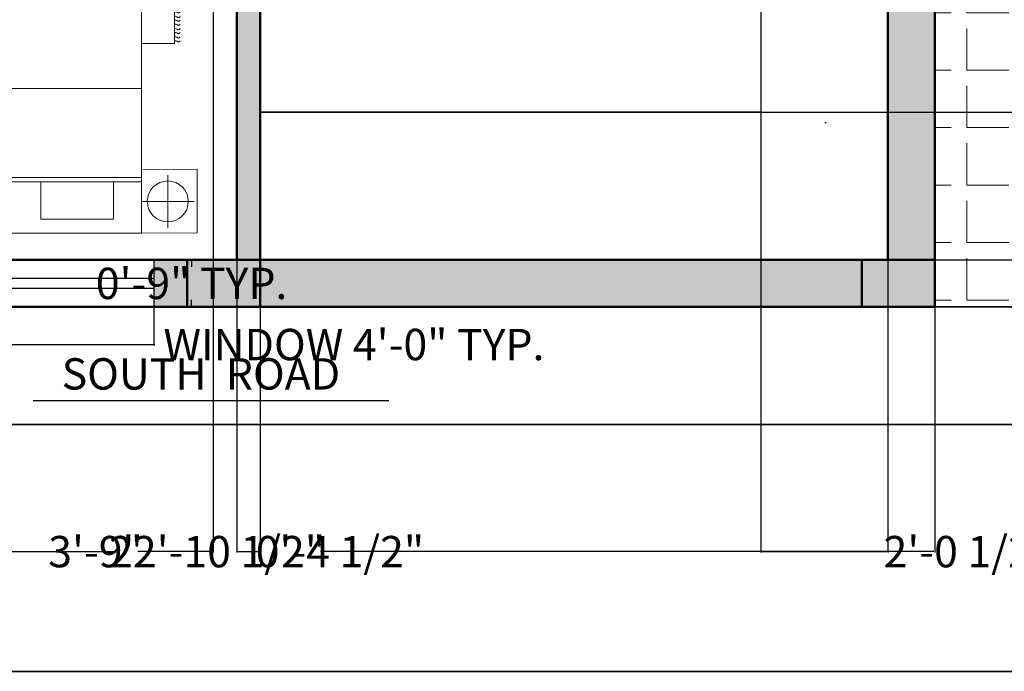
# Model space of a CAD drawing. Units: inches. Extents: x 1601 to 2080, y 5000 to 5589.
# Tile 3 of 11: x 1788 to 1976, y 5000 to 5125. Entities that reach past the tile are written whole.
import ezdxf

# ---------------------------------------------------------------- set-up
doc = ezdxf.new("R2010")
doc.units = ezdxf.units.IN
doc.header["$MEASUREMENT"] = 0
for name, color, linetype, lineweight in [('A-ANNO-DIMS', 2, 'Continuous', 18), ('A-ANNO-TEXT', 7, 'Continuous', 25), ('A-ANNO-TTLB', 7, 'Continuous', 35), ('A-COLS', 7, 'Continuous', 50), ('A-COLS-PATT', 18, 'Continuous', 13), ('A-FLOR-CASE', 8, 'Continuous', 25), ('A-FLOR-PATT', 8, 'Continuous', 13), ('A-FURN', 8, 'Continuous', 18), ('A-GLAZ', 4, 'Continuous', 25), ('A-WALL', 7, 'Continuous', 50), ('A-WALL-PATT', 241, 'Continuous', 13), ('C-PROP', 7, 'Continuous', 35)]:
    doc.layers.add(name, color=color, linetype=linetype, lineweight=lineweight)
doc.styles.get("Standard").update_dxf_attribs({"font": 'arial.ttf'})
doc.dimstyles.get("Standard").update_dxf_attribs({"dimtxt": 6, "dimasz": 0.18, "dimexe": 0.18, "dimexo": 0.0625, "dimgap": 0.09, "dimtad": 0, "dimtih": 1, "dimtoh": 1, "dimdec": 1, "dimzin": 0, "dimdsep": 46, "dimlunit": 3, "dimtxsty": 'Standard', "dimcen": 0.09, "dimadec": 0, "dimazin": 0, "dimtfac": 1, "dimtdec": 1, "dimtofl": 0, "dimtmove": 0, "dimatfit": 3, "dimfxl": 1, "dimtolj": 1, "dimtzin": 0, "dimarcsym": 0})

# ---------------------------------------------------------------- blocks, each defined once
blk = doc.blocks.new('BED-DOUBLE-ENSEMBLE')
for p, q in [((5.6, 61.61), (5.6, 51.56)), ((63.65, 61.72), (63.65, 51.66)), ((10.63, 56.59), (0.57, 56.59)), ((68.68, 56.69), (58.62, 56.69)), ((49.39, 52.82), (10.63, 52.82)), ((49.39, 52.82), (58, 46.47)), ((49.44, 52.82), (49.44, 46.47)), ((49.44, 52), (10.63, 52)), ((49.44, 46.47), (58, 46.47)), ((58.05, 34.96), (10.63, 34.96)), ((4.35, 0), (4.35, 26.37)), ((4.35, 26.37), (10.65, 26.37)), ((58.05, 26.37), (67.59, 26.37)), ((67.59, 26.37), (67.59, 0)), ((67.59, 0), (4.35, 0))]:
    blk.add_line(p, q)
for points in [[(0, 50.39), (10.63, 50.5), (10.63, 62.68), (0, 62.58)], [(58.05, 62.68), (58.05, 11.36), (10.63, 11.36), (10.63, 62.68)], [(58.05, 50.5), (68.68, 50.6), (68.68, 62.78), (58.05, 62.68)], [(29.88, 59.98), (29.88, 52.82), (15.98, 52.82), (15.98, 59.98)], [(49.44, 59.98), (49.44, 52.82), (35.55, 52.82), (35.55, 59.98)]]:
    blk.add_lwpolyline(points, close=True)
for centre in [(5.6, 56.59), (63.65, 56.69)]:
    blk.add_circle(centre, 3.92)
for points, knots in [([(3.23, 25.83), (3.32, 25.96), (3.52, 26.2), (3.86, 25.96), (4.14, 25.78), (4.29, 25.89), (4.35, 25.94)], [0, 0, 0, 0, 0.400747, 0.791423, 1.067667, 1.29709, 1.29709, 1.29709, 1.29709]), ([(3.23, 25.06), (3.32, 25.18), (3.52, 25.42), (3.86, 25.18), (4.14, 25), (4.29, 25.11), (4.35, 25.16)], [0, 0, 0, 0, 0.400747, 0.791423, 1.067667, 1.29709, 1.29709, 1.29709, 1.29709]), ([(3.23, 24.24), (3.32, 24.36), (3.52, 24.6), (3.86, 24.36), (4.14, 24.19), (4.29, 24.3), (4.35, 24.34)], [0, 0, 0, 0, 0.400747, 0.791423, 1.067667, 1.29709, 1.29709, 1.29709, 1.29709]), ([(68.71, 25.83), (68.61, 25.96), (68.42, 26.2), (68.08, 25.96), (67.8, 25.78), (67.65, 25.89), (67.58, 25.94)], [0, 0, 0, 0, 0.400747, 0.791423, 1.067667, 1.29709, 1.29709, 1.29709, 1.29709]), ([(68.71, 25.06), (68.61, 25.18), (68.42, 25.42), (68.08, 25.18), (67.8, 25), (67.65, 25.11), (67.58, 25.16)], [0, 0, 0, 0, 0.400747, 0.791423, 1.067667, 1.29709, 1.29709, 1.29709, 1.29709]), ([(68.71, 24.24), (68.61, 24.36), (68.42, 24.6), (68.08, 24.36), (67.8, 24.19), (67.65, 24.3), (67.58, 24.34)], [0, 0, 0, 0, 0.400747, 0.791423, 1.067667, 1.29709, 1.29709, 1.29709, 1.29709]), ([(3.23, 23.51), (3.32, 23.63), (3.52, 23.87), (3.86, 23.63), (4.14, 23.46), (4.29, 23.57), (4.35, 23.62)], [0, 0, 0, 0, 0.400747, 0.791423, 1.067667, 1.29709, 1.29709, 1.29709, 1.29709]), ([(3.23, 22.63), (3.32, 22.75), (3.52, 22.99), (3.86, 22.75), (4.14, 22.58), (4.29, 22.68), (4.35, 22.73)], [0, 0, 0, 0, 0.400747, 0.791423, 1.067667, 1.29709, 1.29709, 1.29709, 1.29709]), ([(68.71, 23.51), (68.61, 23.63), (68.42, 23.87), (68.08, 23.63), (67.8, 23.46), (67.65, 23.57), (67.58, 23.62)], [0, 0, 0, 0, 0.400747, 0.791423, 1.067667, 1.29709, 1.29709, 1.29709, 1.29709]), ([(68.71, 22.63), (68.61, 22.75), (68.42, 22.99), (68.08, 22.75), (67.8, 22.58), (67.65, 22.68), (67.58, 22.73)], [0, 0, 0, 0, 0.400747, 0.791423, 1.067667, 1.29709, 1.29709, 1.29709, 1.29709]), ([(3.23, 21.88), (3.32, 22), (3.52, 22.24), (3.86, 22), (4.14, 21.83), (4.29, 21.93), (4.35, 21.98)], [0, 0, 0, 0, 0.400747, 0.791423, 1.067667, 1.29709, 1.29709, 1.29709, 1.29709]), ([(3.23, 21.15), (3.32, 21.27), (3.52, 21.51), (3.86, 21.27), (4.14, 21.1), (4.29, 21.2), (4.35, 21.25)], [0, 0, 0, 0, 0.400747, 0.791423, 1.067667, 1.29709, 1.29709, 1.29709, 1.29709]), ([(68.71, 21.88), (68.61, 22), (68.42, 22.24), (68.08, 22), (67.8, 21.83), (67.65, 21.93), (67.58, 21.98)], [0, 0, 0, 0, 0.400747, 0.791423, 1.067667, 1.29709, 1.29709, 1.29709, 1.29709]), ([(68.71, 21.15), (68.61, 21.27), (68.42, 21.51), (68.08, 21.27), (67.8, 21.1), (67.65, 21.2), (67.58, 21.25)], [0, 0, 0, 0, 0.400747, 0.791423, 1.067667, 1.29709, 1.29709, 1.29709, 1.29709]), ([(3.23, 20.27), (3.32, 20.39), (3.52, 20.63), (3.86, 20.39), (4.14, 20.22), (4.29, 20.32), (4.35, 20.37)], [0, 0, 0, 0, 0.400747, 0.791423, 1.067667, 1.29709, 1.29709, 1.29709, 1.29709]), ([(3.23, 19.23), (3.32, 19.35), (3.52, 19.59), (3.86, 19.35), (4.14, 19.18), (4.29, 19.29), (4.35, 19.33)], [0, 0, 0, 0, 0.400747, 0.791423, 1.067667, 1.29709, 1.29709, 1.29709, 1.29709]), ([(68.71, 20.27), (68.61, 20.39), (68.42, 20.63), (68.08, 20.39), (67.8, 20.22), (67.65, 20.32), (67.58, 20.37)], [0, 0, 0, 0, 0.400747, 0.791423, 1.067667, 1.29709, 1.29709, 1.29709, 1.29709]), ([(68.71, 19.23), (68.61, 19.35), (68.42, 19.59), (68.08, 19.35), (67.8, 19.18), (67.65, 19.29), (67.58, 19.33)], [0, 0, 0, 0, 0.400747, 0.791423, 1.067667, 1.29709, 1.29709, 1.29709, 1.29709]), ([(3.23, 18.35), (3.32, 18.47), (3.52, 18.71), (3.86, 18.47), (4.14, 18.3), (4.29, 18.4), (4.35, 18.45)], [0, 0, 0, 0, 0.400747, 0.791423, 1.067667, 1.29709, 1.29709, 1.29709, 1.29709]), ([(3.23, 17.53), (3.32, 17.65), (3.52, 17.89), (3.86, 17.65), (4.14, 17.48), (4.29, 17.59), (4.35, 17.64)], [0, 0, 0, 0, 0.400747, 0.791423, 1.067667, 1.29709, 1.29709, 1.29709, 1.29709]), ([(3.23, 16.76), (3.32, 16.88), (3.52, 17.12), (3.86, 16.88), (4.14, 16.7), (4.29, 16.81), (4.35, 16.86)], [0, 0, 0, 0, 0.400747, 0.791423, 1.067667, 1.29709, 1.29709, 1.29709, 1.29709]), ([(68.71, 18.35), (68.61, 18.47), (68.42, 18.71), (68.08, 18.47), (67.8, 18.3), (67.65, 18.4), (67.58, 18.45)], [0, 0, 0, 0, 0.400747, 0.791423, 1.067667, 1.29709, 1.29709, 1.29709, 1.29709]), ([(68.71, 17.53), (68.61, 17.65), (68.42, 17.89), (68.08, 17.65), (67.8, 17.48), (67.65, 17.59), (67.58, 17.64)], [0, 0, 0, 0, 0.400747, 0.791423, 1.067667, 1.29709, 1.29709, 1.29709, 1.29709]), ([(68.71, 16.76), (68.61, 16.88), (68.42, 17.12), (68.08, 16.88), (67.8, 16.7), (67.65, 16.81), (67.58, 16.86)], [0, 0, 0, 0, 0.400747, 0.791423, 1.067667, 1.29709, 1.29709, 1.29709, 1.29709]), ([(3.23, 15.94), (3.32, 16.06), (3.52, 16.3), (3.86, 16.06), (4.14, 15.89), (4.29, 15.99), (4.35, 16.04)], [0, 0, 0, 0, 0.400747, 0.791423, 1.067667, 1.29709, 1.29709, 1.29709, 1.29709]), ([(3.23, 15.21), (3.32, 15.33), (3.52, 15.57), (3.86, 15.33), (4.14, 15.16), (4.29, 15.27), (4.35, 15.31)], [0, 0, 0, 0, 0.400747, 0.791423, 1.067667, 1.29709, 1.29709, 1.29709, 1.29709]), ([(68.71, 15.94), (68.61, 16.06), (68.42, 16.3), (68.08, 16.06), (67.8, 15.89), (67.65, 15.99), (67.58, 16.04)], [0, 0, 0, 0, 0.400747, 0.791423, 1.067667, 1.29709, 1.29709, 1.29709, 1.29709]), ([(68.71, 15.21), (68.61, 15.33), (68.42, 15.57), (68.08, 15.33), (67.8, 15.16), (67.65, 15.27), (67.58, 15.31)], [0, 0, 0, 0, 0.400747, 0.791423, 1.067667, 1.29709, 1.29709, 1.29709, 1.29709]), ([(3.23, 14.33), (3.32, 14.45), (3.52, 14.69), (3.86, 14.45), (4.14, 14.28), (4.29, 14.38), (4.35, 14.43)], [0, 0, 0, 0, 0.400747, 0.791423, 1.067667, 1.29709, 1.29709, 1.29709, 1.29709]), ([(3.23, 13.58), (3.32, 13.7), (3.52, 13.94), (3.86, 13.7), (4.14, 13.53), (4.29, 13.63), (4.35, 13.68)], [0, 0, 0, 0, 0.400747, 0.791423, 1.067667, 1.29709, 1.29709, 1.29709, 1.29709]), ([(68.71, 14.33), (68.61, 14.45), (68.42, 14.69), (68.08, 14.45), (67.8, 14.28), (67.65, 14.38), (67.58, 14.43)], [0, 0, 0, 0, 0.400747, 0.791423, 1.067667, 1.29709, 1.29709, 1.29709, 1.29709]), ([(68.71, 13.58), (68.61, 13.7), (68.42, 13.94), (68.08, 13.7), (67.8, 13.53), (67.65, 13.63), (67.58, 13.68)], [0, 0, 0, 0, 0.400747, 0.791423, 1.067667, 1.29709, 1.29709, 1.29709, 1.29709]), ([(3.23, 12.85), (3.32, 12.97), (3.52, 13.21), (3.86, 12.97), (4.14, 12.8), (4.29, 12.9), (4.35, 12.95)], [0, 0, 0, 0, 0.400747, 0.791423, 1.067667, 1.29709, 1.29709, 1.29709, 1.29709]), ([(3.23, 11.97), (3.32, 12.09), (3.52, 12.33), (3.86, 12.09), (4.14, 11.92), (4.29, 12.02), (4.35, 12.07)], [0, 0, 0, 0, 0.400747, 0.791423, 1.067667, 1.29709, 1.29709, 1.29709, 1.29709]), ([(68.71, 12.85), (68.61, 12.97), (68.42, 13.21), (68.08, 12.97), (67.8, 12.8), (67.65, 12.9), (67.58, 12.95)], [0, 0, 0, 0, 0.400747, 0.791423, 1.067667, 1.29709, 1.29709, 1.29709, 1.29709]), ([(68.71, 11.97), (68.61, 12.09), (68.42, 12.33), (68.08, 12.09), (67.8, 11.92), (67.65, 12.02), (67.58, 12.07)], [0, 0, 0, 0, 0.400747, 0.791423, 1.067667, 1.29709, 1.29709, 1.29709, 1.29709]), ([(3.23, 10.93), (3.32, 11.05), (3.52, 11.29), (3.86, 11.05), (4.14, 10.88), (4.29, 10.99), (4.35, 11.03)], [0, 0, 0, 0, 0.400747, 0.791423, 1.067667, 1.29709, 1.29709, 1.29709, 1.29709]), ([(3.23, 10.05), (3.32, 10.17), (3.52, 10.41), (3.86, 10.17), (4.14, 10), (4.29, 10.1), (4.35, 10.15)], [0, 0, 0, 0, 0.400747, 0.791423, 1.067667, 1.29709, 1.29709, 1.29709, 1.29709]), ([(3.23, 9.23), (3.32, 9.35), (3.52, 9.59), (3.86, 9.35), (4.14, 9.18), (4.29, 9.29), (4.35, 9.34)], [0, 0, 0, 0, 0.400747, 0.791423, 1.067667, 1.29709, 1.29709, 1.29709, 1.29709]), ([(68.71, 10.93), (68.61, 11.05), (68.42, 11.29), (68.08, 11.05), (67.8, 10.88), (67.65, 10.99), (67.58, 11.03)], [0, 0, 0, 0, 0.400747, 0.791423, 1.067667, 1.29709, 1.29709, 1.29709, 1.29709]), ([(68.71, 10.05), (68.61, 10.17), (68.42, 10.41), (68.08, 10.17), (67.8, 10), (67.65, 10.1), (67.58, 10.15)], [0, 0, 0, 0, 0.400747, 0.791423, 1.067667, 1.29709, 1.29709, 1.29709, 1.29709]), ([(68.71, 9.23), (68.61, 9.35), (68.42, 9.59), (68.08, 9.35), (67.8, 9.18), (67.65, 9.29), (67.58, 9.34)], [0, 0, 0, 0, 0.400747, 0.791423, 1.067667, 1.29709, 1.29709, 1.29709, 1.29709]), ([(3.23, 8.54), (3.32, 8.66), (3.52, 8.9), (3.86, 8.66), (4.14, 8.49), (4.29, 8.6), (4.35, 8.65)], [0, 0, 0, 0, 0.400747, 0.791423, 1.067667, 1.29709, 1.29709, 1.29709, 1.29709]), ([(3.23, 7.73), (3.32, 7.85), (3.52, 8.09), (3.86, 7.85), (4.14, 7.67), (4.29, 7.78), (4.35, 7.83)], [0, 0, 0, 0, 0.400747, 0.791423, 1.067667, 1.29709, 1.29709, 1.29709, 1.29709]), ([(68.71, 8.54), (68.61, 8.66), (68.42, 8.9), (68.08, 8.66), (67.8, 8.49), (67.65, 8.6), (67.58, 8.65)], [0, 0, 0, 0, 0.400747, 0.791423, 1.067667, 1.29709, 1.29709, 1.29709, 1.29709]), ([(68.71, 7.73), (68.61, 7.85), (68.42, 8.09), (68.08, 7.85), (67.8, 7.67), (67.65, 7.78), (67.58, 7.83)], [0, 0, 0, 0, 0.400747, 0.791423, 1.067667, 1.29709, 1.29709, 1.29709, 1.29709]), ([(3.23, 7), (3.32, 7.12), (3.52, 7.36), (3.86, 7.12), (4.14, 6.95), (4.29, 7.05), (4.35, 7.1)], [0, 0, 0, 0, 0.400747, 0.791423, 1.067667, 1.29709, 1.29709, 1.29709, 1.29709]), ([(3.23, 6.12), (3.32, 6.24), (3.52, 6.48), (3.86, 6.24), (4.14, 6.06), (4.29, 6.17), (4.35, 6.22)], [0, 0, 0, 0, 0.400747, 0.791423, 1.067667, 1.29709, 1.29709, 1.29709, 1.29709]), ([(68.71, 7), (68.61, 7.12), (68.42, 7.36), (68.08, 7.12), (67.8, 6.95), (67.65, 7.05), (67.58, 7.1)], [0, 0, 0, 0, 0.400747, 0.791423, 1.067667, 1.29709, 1.29709, 1.29709, 1.29709]), ([(68.71, 6.12), (68.61, 6.24), (68.42, 6.48), (68.08, 6.24), (67.8, 6.06), (67.65, 6.17), (67.58, 6.22)], [0, 0, 0, 0, 0.400747, 0.791423, 1.067667, 1.29709, 1.29709, 1.29709, 1.29709]), ([(3.23, 5.36), (3.32, 5.49), (3.52, 5.72), (3.86, 5.49), (4.14, 5.31), (4.29, 5.42), (4.35, 5.47)], [0, 0, 0, 0, 0.400747, 0.791423, 1.067667, 1.29709, 1.29709, 1.29709, 1.29709]), ([(3.23, 4.64), (3.32, 4.76), (3.52, 5), (3.86, 4.76), (4.14, 4.58), (4.29, 4.69), (4.35, 4.74)], [0, 0, 0, 0, 0.400747, 0.791423, 1.067667, 1.29709, 1.29709, 1.29709, 1.29709]), ([(3.23, 3.75), (3.32, 3.88), (3.52, 4.11), (3.86, 3.88), (4.14, 3.7), (4.29, 3.81), (4.35, 3.86)], [0, 0, 0, 0, 0.400747, 0.791423, 1.067667, 1.29709, 1.29709, 1.29709, 1.29709]), ([(68.71, 5.36), (68.61, 5.49), (68.42, 5.72), (68.08, 5.49), (67.8, 5.31), (67.65, 5.42), (67.58, 5.47)], [0, 0, 0, 0, 0.400747, 0.791423, 1.067667, 1.29709, 1.29709, 1.29709, 1.29709]), ([(68.71, 4.64), (68.61, 4.76), (68.42, 5), (68.08, 4.76), (67.8, 4.59), (67.66, 4.69), (67.59, 4.73)], [0, 0, 0, 0, 0.400747, 0.791423, 1.067667, 1.283686, 1.283686, 1.283686, 1.283686]), ([(68.71, 3.75), (68.61, 3.88), (68.42, 4.11), (68.08, 3.88), (67.8, 3.7), (67.66, 3.8), (67.59, 3.85)], [0, 0, 0, 0, 0.400747, 0.791423, 1.067667, 1.283686, 1.283686, 1.283686, 1.283686]), ([(3.23, 3.32), (3.32, 3.45), (3.51, 3.7), (3.86, 3.44), (4.14, 3.27), (4.29, 3.38), (4.35, 3.43)], [0, 0, 0, 0, 0.407265, 0.802015, 1.07826, 1.307683, 1.307683, 1.307683, 1.307683]), ([(3.23, 2.76), (3.32, 2.88), (3.52, 3.12), (3.86, 2.88), (4.14, 2.71), (4.29, 2.81), (4.35, 2.86)], [0, 0, 0, 0, 0.400747, 0.791423, 1.067667, 1.29709, 1.29709, 1.29709, 1.29709]), ([(3.23, 2.18), (3.32, 2.31), (3.52, 2.54), (3.86, 2.31), (4.14, 2.13), (4.29, 2.24), (4.35, 2.29)], [0, 0, 0, 0, 0.400747, 0.791423, 1.067667, 1.29709, 1.29709, 1.29709, 1.29709]), ([(3.23, 1.88), (3.32, 2), (3.52, 2.24), (3.86, 2), (4.14, 1.82), (4.29, 1.93), (4.35, 1.98)], [0, 0, 0, 0, 0.400747, 0.791423, 1.067667, 1.29709, 1.29709, 1.29709, 1.29709]), ([(68.71, 3.32), (68.61, 3.45), (68.42, 3.69), (68.08, 3.45), (67.8, 3.27), (67.66, 3.38), (67.59, 3.42)], [0, 0, 0, 0, 0.402903, 0.794912, 1.071156, 1.287177, 1.287177, 1.287177, 1.287177]), ([(68.71, 2.73), (68.61, 2.85), (68.42, 3.09), (68.08, 2.85), (67.8, 2.68), (67.66, 2.78), (67.59, 2.82)], [0, 0, 0, 0, 0.400747, 0.791423, 1.067667, 1.283686, 1.283686, 1.283686, 1.283686]), ([(68.71, 2.16), (68.61, 2.28), (68.42, 2.52), (68.08, 2.28), (67.8, 2.11), (67.66, 2.21), (67.59, 2.25)], [0, 0, 0, 0, 0.400747, 0.791423, 1.067667, 1.283686, 1.283686, 1.283686, 1.283686]), ([(68.71, 1.85), (68.61, 1.97), (68.42, 2.21), (68.08, 1.97), (67.8, 1.8), (67.66, 1.9), (67.59, 1.94)], [0, 0, 0, 0, 0.400747, 0.791423, 1.067667, 1.283686, 1.283686, 1.283686, 1.283686]), ([(3.23, 1.46), (3.32, 1.58), (3.52, 1.82), (3.86, 1.58), (4.14, 1.4), (4.29, 1.51), (4.35, 1.56)], [0, 0, 0, 0, 0.400747, 0.791423, 1.067667, 1.29709, 1.29709, 1.29709, 1.29709]), ([(3.23, 1.06), (3.32, 1.18), (3.52, 1.42), (3.86, 1.18), (4.14, 1.01), (4.29, 1.11), (4.35, 1.16)], [0, 0, 0, 0, 0.400747, 0.791423, 1.067667, 1.29709, 1.29709, 1.29709, 1.29709]), ([(3.23, 0.57), (3.32, 0.7), (3.52, 0.93), (3.86, 0.7), (4.14, 0.52), (4.29, 0.63), (4.35, 0.68)], [0, 0, 0, 0, 0.400747, 0.791423, 1.067667, 1.29709, 1.29709, 1.29709, 1.29709]), ([(3.23, 0.07), (3.32, 0.19), (3.52, 0.43), (3.86, 0.19), (4.14, 0.02), (4.29, 0.13), (4.35, 0.18)], [0, 0, 0, 0, 0.400747, 0.791423, 1.067667, 1.29709, 1.29709, 1.29709, 1.29709]), ([(68.71, 1.43), (68.61, 1.55), (68.42, 1.79), (68.08, 1.55), (67.8, 1.38), (67.65, 1.48), (67.58, 1.53)], [0, 0, 0, 0, 0.400747, 0.791423, 1.067667, 1.29709, 1.29709, 1.29709, 1.29709]), ([(68.71, 1.03), (68.61, 1.15), (68.42, 1.39), (68.08, 1.15), (67.8, 0.98), (67.65, 1.09), (67.58, 1.13)], [0, 0, 0, 0, 0.400747, 0.791423, 1.067667, 1.29709, 1.29709, 1.29709, 1.29709]), ([(68.71, 0.55), (68.61, 0.67), (68.42, 0.91), (68.08, 0.67), (67.8, 0.49), (67.65, 0.6), (67.58, 0.65)], [0, 0, 0, 0, 0.400747, 0.791423, 1.067667, 1.29709, 1.29709, 1.29709, 1.29709]), ([(68.71, 0.07), (68.61, 0.19), (68.42, 0.43), (68.08, 0.19), (67.8, 0.02), (67.65, 0.13), (67.58, 0.18)], [0, 0, 0, 0, 0.400747, 0.791423, 1.067667, 1.29709, 1.29709, 1.29709, 1.29709])]:
    blk.add_open_spline(points, degree=3, knots=knots)
blk = doc.blocks.new('WINDOW-48IN')
for p, q in [((0, 0), (0, 9)), ((0, 9), (48, 9)), ((48, 9), (48, 0)), ((0, 5.5), (48, 5.5)), ((48, 3.5), (0, 3.5)), ((48, 0), (0, 0))]:
    blk.add_line(p, q)
blk = doc.blocks.new('*D15')
at = {"layer": 'A-ANNO-DIMS', "color": 0, "lineweight": -2, "transparency": 16777216}
for p, q in [((1765.58, 5069.63), (1765.58, 5062.32)), ((1813.58, 5069.63), (1813.58, 5062.32)), ((1765.76, 5062.5), (1813.4, 5062.5)), ((1813.58, 5062.5), (1813.76, 5062.5))]:
    blk.add_line(p, q, dxfattribs=at)
at = {"layer": 'A-ANNO-DIMS', "color": 0, "transparency": 16777216}
for points in [[(1765.76, 5062.53), (1765.76, 5062.47), (1765.58, 5062.5)], [(1813.4, 5062.53), (1813.4, 5062.47), (1813.58, 5062.5)]]:
    blk.add_solid(points, dxfattribs=at)
at = {"layer": 'Defpoints', "color": 0, "transparency": 16777216}
for p in [(1765.58, 5069.7), (1813.58, 5069.7), (1813.58, 5062.5)]:
    blk.add_point(p, dxfattribs=at)
at = {"layer": 'A-ANNO-DIMS', "color": 0, "transparency": 16777216, "insert": (1851.82, 5062.5), "char_height": 6, "attachment_point": 5}
blk.add_mtext('\\A1;WINDOW 4\'-0" TYP.', dxfattribs=at)
blk = doc.blocks.new('*D16')
at = {"layer": 'A-ANNO-DIMS', "color": 0, "lineweight": -2, "transparency": 16777216}
for p, q in [((1813.65, 5078.7), (1820.96, 5078.7)), ((1820.78, 5078.52), (1820.78, 5077.35)), ((1820.78, 5069.88), (1820.78, 5071.04)), ((1813.65, 5069.7), (1820.96, 5069.7))]:
    blk.add_line(p, q, dxfattribs=at)
at = {"layer": 'A-ANNO-DIMS', "color": 0, "transparency": 16777216}
for points in [[(1820.75, 5078.52), (1820.81, 5078.52), (1820.78, 5078.7)], [(1820.75, 5069.88), (1820.81, 5069.88), (1820.78, 5069.7)]]:
    blk.add_solid(points, dxfattribs=at)
at = {"layer": 'Defpoints', "color": 0, "transparency": 16777216}
for p in [(1813.58, 5078.7), (1820.78, 5078.7), (1813.58, 5069.7)]:
    blk.add_point(p, dxfattribs=at)
at = {"layer": 'A-ANNO-DIMS', "color": 0, "transparency": 16777216, "insert": (1820.78, 5074.2), "char_height": 6, "attachment_point": 5}
blk.add_mtext('\\A1;0\'-9" TYP.', dxfattribs=at)
blk = doc.blocks.new('*D37')
at = {"layer": 'A-ANNO-DIMS', "color": 0, "lineweight": -2, "transparency": 16777216}
for p, q in [((1688.41, 5069.63), (1688.41, 5022.68)), ((1962.91, 5069.63), (1962.91, 5022.68)), ((1688.59, 5022.86), (1805.89, 5022.86)), ((1962.73, 5022.86), (1845.43, 5022.86))]:
    blk.add_line(p, q, dxfattribs=at)
at = {"layer": 'A-ANNO-DIMS', "color": 0, "transparency": 16777216}
for points in [[(1688.59, 5022.89), (1688.59, 5022.83), (1688.41, 5022.86)], [(1962.73, 5022.89), (1962.73, 5022.83), (1962.91, 5022.86)]]:
    blk.add_solid(points, dxfattribs=at)
at = {"layer": 'Defpoints', "color": 0, "transparency": 16777216}
for p in [(1688.41, 5069.7), (1962.91, 5069.7), (1962.91, 5022.86)]:
    blk.add_point(p, dxfattribs=at)
at = {"layer": 'A-ANNO-DIMS', "color": 0, "transparency": 16777216, "insert": (1825.66, 5022.86), "char_height": 6, "attachment_point": 5}
blk.add_mtext('\\A1;22\'-10 1/2"', dxfattribs=at)
blk = doc.blocks.new('*D44')
at = {"layer": 'A-ANNO-DIMS', "color": 0, "lineweight": -2, "transparency": 16777216}
for p, q in [((1929.65, 5106.89), (1929.65, 5022.68)), ((1953.91, 5078.63), (1953.91, 5022.68)), ((1929.83, 5022.86), (1953.73, 5022.86)), ((1953.91, 5022.86), (1954.09, 5022.86))]:
    blk.add_line(p, q, dxfattribs=at)
at = {"layer": 'A-ANNO-DIMS', "color": 0, "transparency": 16777216}
for points in [[(1929.83, 5022.89), (1929.83, 5022.83), (1929.65, 5022.86)], [(1953.73, 5022.89), (1953.73, 5022.83), (1953.91, 5022.86)]]:
    blk.add_solid(points, dxfattribs=at)
at = {"layer": 'Defpoints', "color": 0, "transparency": 16777216}
for p in [(1929.65, 5106.95), (1953.91, 5078.7), (1953.91, 5022.86)]:
    blk.add_point(p, dxfattribs=at)
at = {"layer": 'A-ANNO-DIMS', "color": 0, "transparency": 16777216, "insert": (1969.19, 5022.86), "char_height": 6, "attachment_point": 5}
blk.add_mtext('\\A1;2\'-0 1/2"', dxfattribs=at)
blk = doc.blocks.new('*D45')
at = {"layer": 'A-ANNO-DIMS', "color": 0, "lineweight": -2, "transparency": 16777216}
for p, q in [((1833.97, 5106.95), (2047.44, 5106.95)), ((2047.26, 5106.77), (2047.26, 5096.02)), ((2047.26, 5078.88), (2047.26, 5089.63)), ((1829.47, 5078.7), (2047.44, 5078.7))]:
    blk.add_line(p, q, dxfattribs=at)
at = {"layer": 'A-ANNO-DIMS', "color": 0, "transparency": 16777216}
for points in [[(2047.23, 5106.77), (2047.29, 5106.77), (2047.26, 5106.95)], [(2047.23, 5078.88), (2047.29, 5078.88), (2047.26, 5078.7)]]:
    blk.add_solid(points, dxfattribs=at)
at = {"layer": 'Defpoints', "color": 0, "transparency": 16777216}
for p in [(1833.91, 5106.95), (2047.26, 5106.95), (1829.41, 5078.7)]:
    blk.add_point(p, dxfattribs=at)
at = {"layer": 'A-ANNO-DIMS', "color": 0, "transparency": 16777216, "insert": (2047.26, 5092.83), "char_height": 6, "attachment_point": 5}
blk.add_mtext('\\A1;2\'-4 1/2"', dxfattribs=at)
blk = doc.blocks.new('*D50')
at = {"layer": 'A-ANNO-DIMS', "color": 0, "lineweight": -2, "transparency": 16777216}
for p, q in [((1962.97, 5136.6), (2047.44, 5136.6)), ((2047.26, 5136.42), (2047.26, 5106.29)), ((2047.26, 5069.88), (2047.26, 5100.01)), ((1962.97, 5069.7), (2047.44, 5069.7))]:
    blk.add_line(p, q, dxfattribs=at)
at = {"layer": 'A-ANNO-DIMS', "color": 0, "transparency": 16777216}
for points in [[(2047.23, 5136.42), (2047.29, 5136.42), (2047.26, 5136.6)], [(2047.23, 5069.88), (2047.29, 5069.88), (2047.26, 5069.7)]]:
    blk.add_solid(points, dxfattribs=at)
at = {"layer": 'Defpoints', "color": 0, "transparency": 16777216}
for p in [(1962.91, 5136.6), (2047.26, 5136.6), (1962.91, 5069.7)]:
    blk.add_point(p, dxfattribs=at)
at = {"layer": 'A-ANNO-DIMS', "color": 0, "transparency": 16777216, "insert": (2047.26, 5103.15), "char_height": 6, "attachment_point": 5}
blk.add_mtext('\\A1;5\'-7"', dxfattribs=at)
blk = doc.blocks.new('*D57')
at = {"layer": 'A-ANNO-DIMS', "color": 0, "lineweight": -2, "transparency": 16777216}
for p, q in [((1829.41, 5244.58), (1829.41, 5022.68)), ((1833.91, 5244.58), (1833.91, 5022.68)), ((1829.59, 5022.86), (1833.73, 5022.86)), ((1833.91, 5022.86), (1834.09, 5022.86))]:
    blk.add_line(p, q, dxfattribs=at)
at = {"layer": 'A-ANNO-DIMS', "color": 0, "transparency": 16777216}
for points in [[(1829.59, 5022.89), (1829.59, 5022.83), (1829.41, 5022.86)], [(1833.73, 5022.89), (1833.73, 5022.83), (1833.91, 5022.86)]]:
    blk.add_solid(points, dxfattribs=at)
at = {"layer": 'Defpoints', "color": 0, "transparency": 16777216}
for p in [(1829.41, 5244.64), (1833.91, 5244.64), (1833.91, 5022.86)]:
    blk.add_point(p, dxfattribs=at)
at = {"layer": 'A-ANNO-DIMS', "color": 0, "transparency": 16777216, "insert": (1849.14, 5022.86), "char_height": 6, "attachment_point": 5}
blk.add_mtext('\\A1;0\'-4 1/2"', dxfattribs=at)
blk = doc.blocks.new('*D58')
at = {"layer": 'A-ANNO-DIMS', "color": 0, "lineweight": -2, "transparency": 16777216}
for p, q in [((1779.91, 5209.13), (1779.91, 5022.68)), ((1824.91, 5209.13), (1824.91, 5022.68)), ((1780.09, 5022.86), (1794.35, 5022.86)), ((1824.73, 5022.86), (1810.47, 5022.86))]:
    blk.add_line(p, q, dxfattribs=at)
at = {"layer": 'A-ANNO-DIMS', "color": 0, "transparency": 16777216}
for points in [[(1780.09, 5022.89), (1780.09, 5022.83), (1779.91, 5022.86)], [(1824.73, 5022.89), (1824.73, 5022.83), (1824.91, 5022.86)]]:
    blk.add_solid(points, dxfattribs=at)
at = {"layer": 'Defpoints', "color": 0, "transparency": 16777216}
for p in [(1779.91, 5209.2), (1824.91, 5209.2), (1824.91, 5022.86)]:
    blk.add_point(p, dxfattribs=at)
at = {"layer": 'A-ANNO-DIMS', "color": 0, "transparency": 16777216, "insert": (1802.41, 5022.86), "char_height": 6, "attachment_point": 5}
blk.add_mtext('\\A1;3\'-9"', dxfattribs=at)
blk = doc.blocks.new('*D64')
at = {"layer": 'A-ANNO-DIMS', "color": 0, "lineweight": -2, "transparency": 16777216}
for p, q in [((1941.65, 5182.17), (1941.83, 5182.17)), ((1941.83, 5182.17), (1941.89, 5153.4)), ((1941.91, 5104.96), (1942.09, 5104.96)), ((1942, 5104.87), (1942, 5105.05))]:
    blk.add_line(p, q, dxfattribs=at)
at = {"layer": 'A-ANNO-DIMS', "color": 0, "transparency": 16777216}
blk.add_solid([(1941.92, 5153.4), (1941.86, 5153.4), (1941.89, 5153.22)], dxfattribs=at)
at = {"layer": 'Defpoints', "color": 0, "transparency": 16777216}
for p in [(1941.89, 5153.22), (1942, 5104.96)]:
    blk.add_point(p, dxfattribs=at)
at = {"layer": 'A-ANNO-DIMS', "color": 0, "transparency": 16777216, "insert": (1917.23, 5182.17), "char_height": 6, "attachment_point": 5}
blk.add_mtext('\\A1;2X R4\'-0 1/2"', dxfattribs=at)

msp = doc.modelspace()

# ---------------------------------------------------------------- hatches: boundary and pattern name
at = {"layer": 'A-COLS-PATT'}
h = msp.add_hatch(color=256, dxfattribs=at)
h.dxf.hatch_style = 1
h.paths.add_polyline_path([(1702.41, 5431.2), (1688.41, 5431.2), (1688.41, 5422.2), (1702.41, 5422.2)])
h.paths.add_polyline_path([(1836.17, 5431.2), (1822.17, 5431.2), (1822.17, 5422.2), (1836.17, 5422.2)])
h.paths.add_polyline_path([(1962.91, 5431.2), (1948.91, 5431.2), (1948.91, 5422.2), (1962.91, 5422.2)])
h.paths.add_polyline_path([(1697.41, 5314.2), (1688.41, 5314.2), (1688.41, 5300.2), (1697.41, 5300.2)])
h.paths.add_polyline_path([(1833.91, 5314.2), (1824.91, 5314.2), (1824.91, 5300.2), (1833.91, 5300.2)])
h.paths.add_polyline_path([(1962.91, 5314.2), (1953.91, 5314.2), (1953.91, 5300.2), (1962.91, 5300.2)])
h.paths.add_polyline_path([(1697.41, 5209.2), (1688.41, 5209.2), (1688.41, 5195.2), (1697.41, 5195.2)])
h.paths.add_polyline_path([(1833.91, 5209.2), (1824.91, 5209.2), (1824.91, 5195.2), (1833.91, 5195.2)])
h.paths.add_polyline_path([(1962.91, 5209.2), (1953.91, 5209.2), (1953.91, 5195.2), (1962.91, 5195.2)])
h.paths.add_polyline_path([(1697.41, 5083.7), (1688.41, 5083.7), (1688.41, 5069.7), (1697.41, 5069.7)])
h.paths.add_polyline_path([(1833.91, 5078.7), (1819.91, 5078.7), (1819.91, 5069.7), (1833.91, 5069.7)])
h.paths.add_polyline_path([(1962.91, 5078.7), (1948.91, 5078.7), (1948.91, 5069.7), (1962.91, 5069.7)])
at = {"layer": 'A-FLOR-PATT'}
h = msp.add_hatch(dxfattribs=at)
h.set_pattern_fill('ANGLE', color=256, scale=40)
h.set_pattern_definition([(0, (0, 0), (0, 11), [8, -3]), (90, (0, 0), (-11, 7e-16), [8, -3])])
h.paths.add_polyline_path([(2022.91, 5509.2), (1941.91, 5509.2), (1911.91, 5509.2), (1864.41, 5509.2), (1864.41, 5489.7), (1868.54, 5489.7, -0.022155), (1868.52, 5490.01, -1), (1875.53, 5490.01, -0.956651), (1868.54, 5489.7), (1864.41, 5489.7), (1864.41, 5470.2), (1794.41, 5470.2), (1794.41, 5431.2), (1811.95, 5431.2), (1911.91, 5431.2), (1941.91, 5431.2), (1942.91, 5431.2), (1945.91, 5431.2), (1948.91, 5431.2), (1962.91, 5431.2), (1962.91, 5415.29), (1962.91, 5385.29), (1962.91, 5384.29), (1962.91, 5381.29), (1962.91, 5333.29), (1962.91, 5069.7), (2022.91, 5069.7)])
h.paths.add_polyline_path([(2000.28, 5267.55), (2000.28, 5367.64), (1987.91, 5367.64), (1987.91, 5267.55)], flags=24)
h.paths.add_polyline_path([(1879.42, 5455.52), (1969.04, 5455.52), (1969.04, 5467.88), (1879.42, 5467.88)], flags=24)
at = {"layer": 'A-WALL-PATT'}
h = msp.add_hatch(color=256, dxfattribs=at)
h.dxf.hatch_style = 1
h.paths.add_polyline_path([(1763.95, 5431.2), (1702.41, 5431.2), (1702.41, 5422.2), (1763.95, 5422.2)])
h.paths.add_polyline_path([(1697.41, 5422.2), (1688.41, 5422.2), (1688.41, 5314.2), (1697.41, 5314.2)])
h.paths.add_polyline_path([(1740.41, 5314.2), (1697.41, 5314.2), (1697.41, 5309.7), (1740.41, 5309.7)], flags=17)
h.paths.add_polyline_path([(1822.17, 5431.2), (1811.95, 5431.2), (1811.95, 5422.2), (1822.17, 5422.2)])
h.paths.add_polyline_path([(1845.52, 5431.2), (1836.17, 5431.2), (1836.17, 5422.2), (1845.52, 5422.2)])
h.paths.add_polyline_path([(1910.91, 5431.2), (1881.52, 5431.2), (1881.52, 5422.2), (1910.91, 5422.2)])
h.paths.add_polyline_path([(1948.91, 5431.2), (1945.91, 5431.2), (1942.91, 5431.2), (1942.91, 5422.2), (1948.91, 5422.2)])
h.paths.add_polyline_path([(1962.91, 5422.2), (1953.91, 5422.2), (1953.91, 5416.29), (1962.91, 5416.29)])
h.paths.add_polyline_path([(1962.91, 5384.29), (1953.91, 5384.29), (1953.91, 5381.29), (1962.91, 5381.29)])
h.paths.add_polyline_path([(1962.91, 5333.29), (1953.91, 5333.29), (1953.91, 5314.2), (1962.91, 5314.2)])
h.paths.add_polyline_path([(1962.91, 5300.2), (1953.91, 5300.2), (1953.91, 5236.2), (1875.91, 5236.2), (1875.91, 5230.7), (1881.91, 5230.7), (1881.91, 5231.7), (1953.91, 5231.7), (1953.91, 5219.2), (1962.91, 5219.2)])
h.paths.add_polyline_path([(1962.91, 5185.2), (1953.91, 5185.2), (1953.91, 5183.7), (1881.91, 5183.7), (1881.91, 5184.7), (1875.91, 5184.7), (1875.91, 5183.7), (1875.91, 5179.2), (1953.91, 5179.2), (1953.91, 5172.6), (1962.91, 5172.6)])
h.paths.add_polyline_path([(1962.91, 5136.6), (1953.91, 5136.6), (1953.91, 5078.7), (1962.91, 5078.7)])
h.paths.add_polyline_path([(1948.91, 5078.7), (1833.91, 5078.7), (1833.91, 5069.7), (1948.91, 5069.7)])
h.paths.add_polyline_path([(1833.91, 5195.2), (1829.41, 5195.2), (1829.41, 5078.7), (1833.91, 5078.7)])
h.paths.add_polyline_path([(1819.91, 5078.7), (1813.58, 5078.7), (1813.58, 5069.7), (1819.91, 5069.7)])
h.paths.add_polyline_path([(1765.58, 5078.7), (1697.41, 5078.7), (1697.41, 5069.7), (1765.58, 5069.7)])
h.paths.add_polyline_path([(1697.41, 5195.2), (1688.41, 5195.2), (1688.41, 5083.7), (1697.41, 5083.7)])
h.paths.add_polyline_path([(1740.41, 5209.2), (1697.41, 5209.2), (1697.41, 5204.7), (1740.41, 5204.7)], flags=17)
h.paths.add_polyline_path([(1787.91, 5209.2), (1779.91, 5209.2), (1779.91, 5309.7), (1787.91, 5309.7), (1787.91, 5314.2), (1772.41, 5314.2), (1772.41, 5309.7), (1775.41, 5309.7), (1775.41, 5261.7), (1697.41, 5261.7), (1697.41, 5273.07), (1688.41, 5273.07), (1688.41, 5242.37), (1697.41, 5242.37), (1697.41, 5257.2), (1775.41, 5257.2), (1775.41, 5209.2), (1772.41, 5209.2), (1772.41, 5204.7), (1775.41, 5204.7), (1787.91, 5204.7)])
h.paths.add_polyline_path([(1697.41, 5218.37), (1688.41, 5218.37), (1688.41, 5209.2), (1697.41, 5209.2)], flags=17)
h.paths.add_polyline_path([(1833.91, 5422.2), (1829.41, 5422.2), (1829.41, 5314.2), (1833.91, 5314.2)])
h.paths.add_polyline_path([(1697.41, 5300.2), (1688.41, 5300.2), (1688.41, 5297.07), (1697.41, 5297.07)], flags=17)

# ---------------------------------------------------------------- linework, layer by layer
at = {"layer": 'A-ANNO-TEXT'}
msp.add_line((1790.47, 5051.81), (1858.52, 5051.81), dxfattribs=at)
at = {"layer": 'A-ANNO-TTLB'}
msp.add_lwpolyline([(1600.55, 5589.45), (2079.72, 5589.45), (2079.72, 4999.95), (1600.55, 4999.95)], close=True, dxfattribs=at)
at = {"layer": 'A-COLS'}
for p, q in [((1819.91, 5078.7), (1819.91, 5069.7)), ((1948.91, 5078.7), (1948.91, 5069.7))]:
    msp.add_line(p, q, dxfattribs=at)
at = {"layer": 'A-FLOR-CASE'}
for p, q in [((1929.65, 5174.81), (1929.65, 5106.95)), ((1929.65, 5106.95), (1833.91, 5106.95))]:
    msp.add_line(p, q, dxfattribs=at)
at = {"layer": 'A-WALL'}
for p, q in [((1962.91, 5385.29), (1962.91, 5069.7)), ((1833.91, 5244.64), (1833.91, 5069.7)), ((1829.41, 5195.2), (1829.41, 5078.7)), ((1953.91, 5179.2), (1953.91, 5078.7)), ((1697.41, 5078.7), (1962.91, 5078.7)), ((1688.41, 5069.7), (1962.91, 5069.7))]:
    msp.add_line(p, q, dxfattribs=at)
at = {"layer": 'C-PROP'}
for p, q in [((2022.91, 5069.7), (1962.91, 5069.7)), ((1664.41, 5047.21), (2022.91, 5047.21))]:
    msp.add_line(p, q, dxfattribs=at)

# ---------------------------------------------------------------- block references
at = {"layer": 'A-FURN', "rotation": 180}
msp.add_blockref('BED-DOUBLE-ENSEMBLE', (1821.83, 5146.47), dxfattribs=at)
at = {"layer": 'A-GLAZ'}
msp.add_blockref('WINDOW-48IN', (1765.58, 5069.7), dxfattribs=at)

# ---------------------------------------------------------------- texts
at = {"layer": 'A-ANNO-TEXT', "insert": (1795.93, 5059.88), "char_height": 6, "attachment_point": 1}
msp.add_mtext_dynamic_manual_height_columns('SOUTH  ROAD', width=70.8814, gutter_width=30, heights=[0], dxfattribs=at)

# ---------------------------------------------------------------- dimensions: what is measured, and where the dimension line sits
at = {"layer": 'A-ANNO-DIMS'}
for base, p1, p2, picture, middle in [((1833.91, 5022.86), (1829.41, 5244.64), (1833.91, 5244.64), '*D57', (1849.14, 5022.86)), ((1824.91, 5022.86), (1779.91, 5209.2), (1824.91, 5209.2), '*D58', (1802.41, 5022.86)), ((1953.91, 5022.86), (1929.65, 5106.95), (1953.91, 5078.7), '*D44', (1969.19, 5022.86)), ((1962.91, 5022.86), (1688.41, 5069.7), (1962.91, 5069.7), '*D37', (1825.66, 5022.86))]:
    dim = msp.add_linear_dim(base=base, p1=p1, p2=p2, dimstyle='Standard', override={"dimdec": 1, "dimlfac": 1, "dimrnd": 0, "dimzin": 1, "dimdsep": 46, "dimlunit": 4, "dimfrac": 2}, dxfattribs=at)
    dim.commit()
    dim.dimension.update_dxf_attribs({"geometry": picture, "text_midpoint": middle})
dim = msp.add_radius_dim(center=(1942, 5104.96), mpoint=(1941.89, 5153.22), text='2X <>', dimstyle='Standard', override={"dimdec": 1, "dimlfac": 1, "dimrnd": 0, "dimzin": 1, "dimdsep": 46, "dimlunit": 4, "dimfrac": 2}, dxfattribs=at)
dim.commit()
dim.dimension.update_dxf_attribs({"geometry": '*D64', "text_midpoint": (1917.23, 5182.17), "dimtype": 164})
for base, p1, p2, picture, middle in [((2047.26, 5136.6), (1962.91, 5069.7), (1962.91, 5136.6), '*D50', (2047.26, 5103.15)), ((2047.2582, 5106.9548), (1829.4082, 5078.6964), (1833.9082, 5106.9548), '*D45', (2047.2582, 5092.8256))]:
    dim = msp.add_linear_dim(base=base, p1=p1, p2=p2, angle=90, dimstyle='Standard', override={"dimdec": 1, "dimlfac": 1, "dimrnd": 0, "dimzin": 1, "dimdsep": 46, "dimlunit": 4, "dimfrac": 2}, dxfattribs=at)
    dim.commit()
    dim.dimension.update_dxf_attribs({"geometry": picture, "text_midpoint": middle})
dim = msp.add_linear_dim(base=(1820.78, 5078.7), p1=(1813.58, 5069.7), p2=(1813.58, 5078.7), angle=90, text='<> TYP.', dimstyle='Standard', override={"dimdec": 1, "dimlfac": 1, "dimrnd": 0, "dimzin": 1, "dimdsep": 46, "dimlunit": 4, "dimfrac": 2}, dxfattribs=at)
dim.commit()
dim.dimension.update_dxf_attribs({"geometry": '*D16', "text_midpoint": (1820.78, 5074.2)})
dim = msp.add_linear_dim(base=(1813.58, 5062.5), p1=(1765.58, 5069.7), p2=(1813.58, 5069.7), text='WINDOW <> TYP.', dimstyle='Standard', override={"dimdec": 1, "dimlfac": 1, "dimrnd": 0, "dimzin": 1, "dimdsep": 46, "dimlunit": 4, "dimfrac": 2}, dxfattribs=at)
dim.commit()
dim.dimension.update_dxf_attribs({"geometry": '*D15', "text_midpoint": (1851.82, 5062.5)})

doc.saveas('drawing.dxf')
